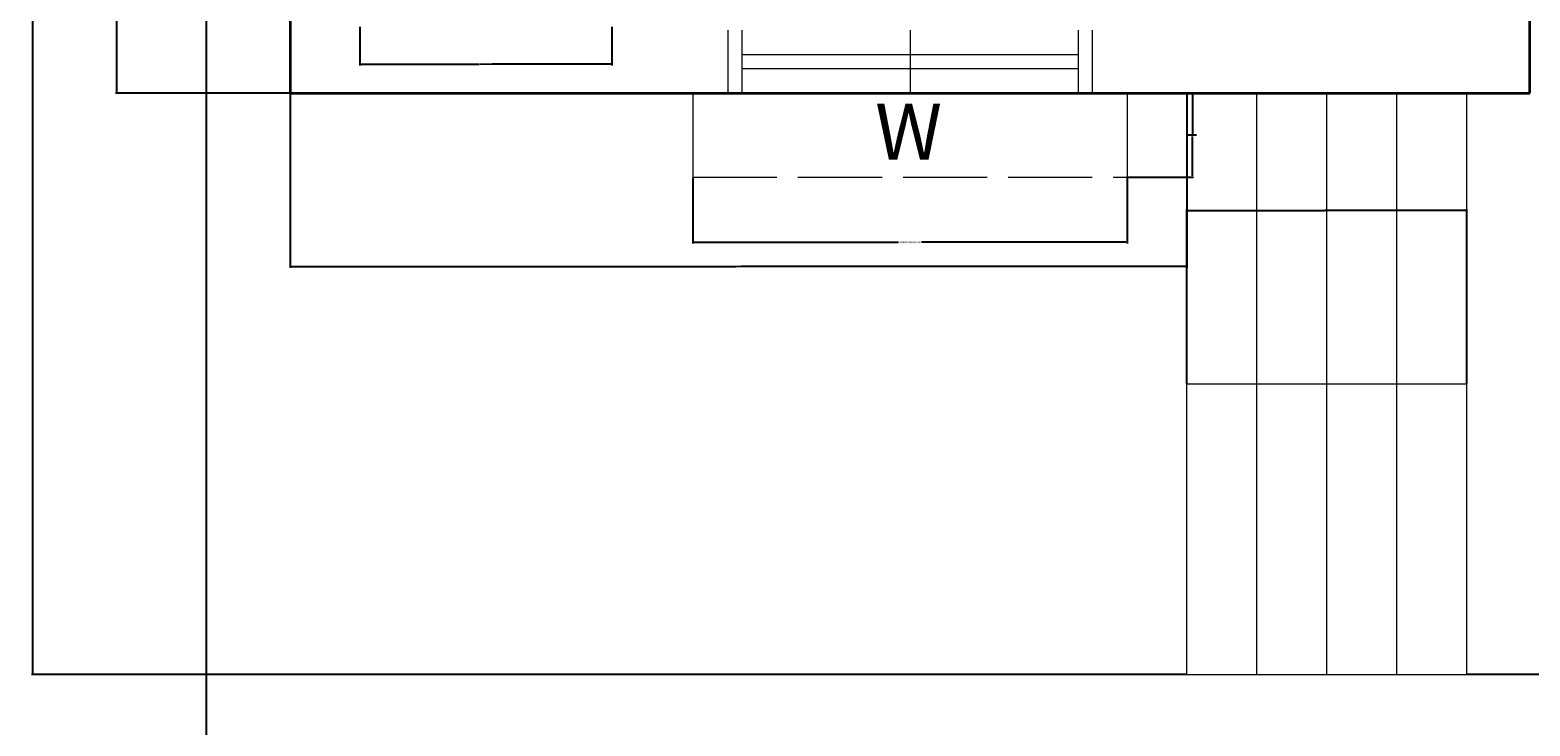
# Model space of a CAD drawing. Units: inches. Extents: x -35 to 832, y -515 to 219.
# Tile 2 of 7: x -35 to 179, y -262 to -163. Entities that reach past the tile are written whole.
import ezdxf

# ---------------------------------------------------------------- set-up
doc = ezdxf.new("R2010")
doc.units = ezdxf.units.IN
doc.header["$MEASUREMENT"] = 0
doc.linetypes.add('ACAD_ISO02W100', pattern=[15, 12, -3])
for name, color, linetype, lineweight in [('A-ANNO-TEXT', 7, 'Continuous', 18), ('A-FLOR', 7, 'Continuous', 25), ('A-FLOR-STRS', 2, 'Continuous', 18), ('A-GLAZ', 2, 'Continuous', 18), ('A-GLAZ-OVHD', 2, 'ACAD_ISO02W100', 13), ('A-WALL', 10, 'Continuous', 35), ('S-ANNO-DIMS', 2, 'Continuous', 18)]:
    doc.layers.add(name, color=color, linetype=linetype, lineweight=lineweight)
doc.styles.get("Standard").update_dxf_attribs({"font": 'arial.ttf'})
doc.dimstyles.get("Standard").update_dxf_attribs({"dimtxt": 0.18, "dimasz": 0.18, "dimexe": 0.18, "dimexo": 0.0625, "dimgap": 0.09, "dimtad": 0, "dimtih": 1, "dimtoh": 1, "dimdec": 1, "dimzin": 0, "dimdsep": 46, "dimlunit": 4, "dimtxsty": 'Standard', "dimcen": 0.09, "dimclrd": 211, "dimclre": 4, "dimclrt": 3, "dimadec": 0, "dimazin": 0, "dimtfac": 0.5, "dimtdec": 1, "dimtofl": 0, "dimtmove": 0, "dimatfit": 3, "dimfxl": 1, "dimtfill": 2, "dimtfillclr": 61, "dimtolj": 1, "dimtzin": 0, "dimarcsym": 0})

# ---------------------------------------------------------------- blocks, each defined once
blk = doc.blocks.new('WIN-48')
for p, q in [((0, 9), (0, 0)), ((2, 9), (2, 0)), ((26, 9), (26, 0)), ((50, 9), (50, 0)), ((52, 9), (52, 0)), ((2, 5.5), (50, 5.5)), ((2, 3.5), (50, 3.5))]:
    blk.add_line(p, q)
blk = doc.blocks.new('WIN-48-HOOD')
for p, q in [((5, 12), (0, 12)), ((0, 12), (0, 0)), ((57, 12), (62, 12)), ((62, 12), (62, 0)), ((0, 0), (62, 0))]:
    blk.add_line(p, q)
blk = doc.blocks.new('*D63')
at = {"layer": 'Defpoints', "color": 0, "transparency": 16777216}
for p in [(59.3, -183.95), (121.3, -183.95), (121.3, -193.25)]:
    blk.add_point(p, dxfattribs=at)
at = {"layer": 'S-ANNO-DIMS', "color": 4, "lineweight": -2, "transparency": 16777216}
for p, q in [((59.3, -184.01), (59.3, -193.43)), ((121.3, -184.01), (121.3, -193.43))]:
    blk.add_line(p, q, dxfattribs=at)
at = {"layer": 'S-ANNO-DIMS', "color": 211, "lineweight": -2, "transparency": 16777216}
for p, q in [((59.48, -193.25), (88.66, -193.25)), ((121.12, -193.25), (91.94, -193.25))]:
    blk.add_line(p, q, dxfattribs=at)
at = {"layer": 'S-ANNO-DIMS', "color": 211, "transparency": 16777216}
for points in [[(59.48, -193.22), (59.48, -193.28), (59.3, -193.25)], [(121.12, -193.22), (121.12, -193.28), (121.3, -193.25)]]:
    blk.add_solid(points, dxfattribs=at)
at = {"layer": 'S-ANNO-DIMS', "color": 3, "transparency": 16777216, "insert": (90.3, -193.25), "char_height": 0.18, "attachment_point": 5, "bg_fill": 1, "box_fill_scale": 1.25, "bg_fill_color": 61, "bg_fill_transparency": 0}
blk.add_mtext('\\A1;WINDOW HOOD 5\'-2" TYP.', dxfattribs=at)
blk = doc.blocks.new('*D64')
at = {"layer": 'Defpoints', "color": 0, "transparency": 16777216}
for p in [(121.3, -171.95), (130.6, -171.95), (121.3, -183.95)]:
    blk.add_point(p, dxfattribs=at)
at = {"layer": 'S-ANNO-DIMS', "color": 4, "lineweight": -2, "transparency": 16777216}
for p, q in [((121.36, -171.95), (130.78, -171.95)), ((121.36, -183.95), (130.78, -183.95))]:
    blk.add_line(p, q, dxfattribs=at)
at = {"layer": 'S-ANNO-DIMS', "color": 211, "lineweight": -2, "transparency": 16777216}
for p, q in [((130.6, -172.13), (130.6, -177.77)), ((130.6, -183.77), (130.6, -178.13))]:
    blk.add_line(p, q, dxfattribs=at)
at = {"layer": 'S-ANNO-DIMS', "color": 211, "transparency": 16777216}
for points in [[(130.57, -172.13), (130.63, -172.13), (130.6, -171.95)], [(130.57, -183.77), (130.63, -183.77), (130.6, -183.95)]]:
    blk.add_solid(points, dxfattribs=at)
at = {"layer": 'S-ANNO-DIMS', "color": 3, "transparency": 16777216, "insert": (130.6, -177.95), "char_height": 0.18, "attachment_point": 5, "bg_fill": 1, "box_fill_scale": 1.25, "bg_fill_color": 61, "bg_fill_transparency": 0}
blk.add_mtext('\\A1;1\'-0" TYP.', dxfattribs=at)
blk = doc.blocks.new('*D81')
at = {"layer": 'Defpoints', "color": 0, "transparency": 16777216}
for p in [(11.74, -162.42), (47.74, -162.42), (47.74, -167.82)]:
    blk.add_point(p, dxfattribs=at)
at = {"layer": 'S-ANNO-DIMS', "color": 4, "lineweight": -2, "transparency": 16777216}
for p, q in [((11.74, -162.48), (11.74, -168)), ((47.74, -162.48), (47.74, -168))]:
    blk.add_line(p, q, dxfattribs=at)
at = {"layer": 'S-ANNO-DIMS', "color": 211, "lineweight": -2, "transparency": 16777216}
for p, q in [((11.92, -167.82), (28.83, -167.82)), ((47.56, -167.82), (30.65, -167.82))]:
    blk.add_line(p, q, dxfattribs=at)
at = {"layer": 'S-ANNO-DIMS', "color": 211, "transparency": 16777216}
for points in [[(11.92, -167.79), (11.92, -167.85), (11.74, -167.82)], [(47.56, -167.79), (47.56, -167.85), (47.74, -167.82)]]:
    blk.add_solid(points, dxfattribs=at)
at = {"layer": 'S-ANNO-DIMS', "color": 3, "transparency": 16777216, "insert": (29.74, -167.82), "char_height": 0.18, "attachment_point": 5, "bg_fill": 1, "box_fill_scale": 1.25, "bg_fill_color": 61, "bg_fill_transparency": 0}
blk.add_mtext('\\A1;CABINET 3\'-0"', dxfattribs=at)
blk = doc.blocks.new('*D107')
at = {"layer": 'Defpoints', "color": 0, "transparency": 16777216}
for p in [(1.8, -171.95), (129.8, -171.95), (1.8, -196.7)]:
    blk.add_point(p, dxfattribs=at)
at = {"layer": 'S-ANNO-DIMS', "color": 4, "lineweight": -2, "transparency": 16777216}
for p, q in [((1.8, -172.01), (1.8, -196.88)), ((129.8, -172.01), (129.8, -196.88))]:
    blk.add_line(p, q, dxfattribs=at)
at = {"layer": 'S-ANNO-DIMS', "color": 211, "lineweight": -2, "transparency": 16777216}
for p, q in [((1.98, -196.7), (65.41, -196.7)), ((129.62, -196.7), (66.19, -196.7))]:
    blk.add_line(p, q, dxfattribs=at)
at = {"layer": 'S-ANNO-DIMS', "color": 211, "transparency": 16777216}
for points in [[(1.98, -196.67), (1.98, -196.73), (1.8, -196.7)], [(129.62, -196.67), (129.62, -196.73), (129.8, -196.7)]]:
    blk.add_solid(points, dxfattribs=at)
at = {"layer": 'S-ANNO-DIMS', "color": 3, "transparency": 16777216, "insert": (65.8, -196.7), "char_height": 0.18, "attachment_point": 5, "bg_fill": 1, "box_fill_scale": 1.25, "bg_fill_color": 61, "bg_fill_transparency": 0}
blk.add_mtext('\\A1;10\'-8"', dxfattribs=at)
blk = doc.blocks.new('*D108')
at = {"layer": 'Defpoints', "color": 0, "transparency": 16777216}
for p in [(169.8, -188.7), (129.8, -213.45), (169.8, -213.45)]:
    blk.add_point(p, dxfattribs=at)
at = {"layer": 'S-ANNO-DIMS', "color": 4, "lineweight": -2, "transparency": 16777216}
for p, q in [((129.8, -213.39), (129.8, -188.52)), ((169.8, -213.39), (169.8, -188.52))]:
    blk.add_line(p, q, dxfattribs=at)
at = {"layer": 'S-ANNO-DIMS', "color": 211, "lineweight": -2, "transparency": 16777216}
for p, q in [((129.98, -188.7), (149.47, -188.7)), ((169.62, -188.7), (150.13, -188.7))]:
    blk.add_line(p, q, dxfattribs=at)
at = {"layer": 'S-ANNO-DIMS', "color": 211, "transparency": 16777216}
for points in [[(129.98, -188.67), (129.98, -188.73), (129.8, -188.7)], [(169.62, -188.67), (169.62, -188.73), (169.8, -188.7)]]:
    blk.add_solid(points, dxfattribs=at)
at = {"layer": 'S-ANNO-DIMS', "color": 3, "transparency": 16777216, "insert": (149.8, -188.7), "char_height": 0.18, "attachment_point": 5, "bg_fill": 1, "box_fill_scale": 1.25, "bg_fill_color": 61, "bg_fill_transparency": 0}
blk.add_mtext('\\A1;3\'-4"', dxfattribs=at)
blk = doc.blocks.new('*D109')
at = {"layer": 'Defpoints', "color": 0, "transparency": 16777216}
for p in [(365.8, -100.95), (-10.2, -143.45), (365.8, -279.7)]:
    blk.add_point(p, dxfattribs=at)
at = {"layer": 'S-ANNO-DIMS', "color": 4, "lineweight": -2, "transparency": 16777216}
for p, q in [((365.8, -101.01), (365.8, -279.88)), ((-10.2, -143.51), (-10.2, -279.88))]:
    blk.add_line(p, q, dxfattribs=at)
at = {"layer": 'S-ANNO-DIMS', "color": 211, "lineweight": -2, "transparency": 16777216}
for p, q in [((-10.02, -279.7), (177.4, -279.7)), ((365.62, -279.7), (178.2, -279.7))]:
    blk.add_line(p, q, dxfattribs=at)
at = {"layer": 'S-ANNO-DIMS', "color": 211, "transparency": 16777216}
for points in [[(-10.02, -279.67), (-10.02, -279.73), (-10.2, -279.7)], [(365.62, -279.67), (365.62, -279.73), (365.8, -279.7)]]:
    blk.add_solid(points, dxfattribs=at)
at = {"layer": 'S-ANNO-DIMS', "color": 3, "transparency": 16777216, "insert": (177.8, -279.7), "char_height": 0.18, "attachment_point": 5, "bg_fill": 1, "box_fill_scale": 1.25, "bg_fill_color": 61, "bg_fill_transparency": 0}
blk.add_mtext('\\A1;31\'-4"', dxfattribs=at)
blk = doc.blocks.new('*D110')
at = {"layer": 'Defpoints', "color": 0, "transparency": 16777216}
for p in [(59.3, 194.05), (-34.95, -254.95), (129.8, -254.95)]:
    blk.add_point(p, dxfattribs=at)
at = {"layer": 'S-ANNO-DIMS', "color": 4, "lineweight": -2, "transparency": 16777216}
for p, q in [((59.24, 194.05), (-35.13, 194.05)), ((129.74, -254.95), (-35.13, -254.95))]:
    blk.add_line(p, q, dxfattribs=at)
at = {"layer": 'S-ANNO-DIMS', "color": 211, "lineweight": -2, "transparency": 16777216}
for p, q in [((-34.95, 193.87), (-34.95, -30.27)), ((-34.95, -254.77), (-34.95, -30.63))]:
    blk.add_line(p, q, dxfattribs=at)
at = {"layer": 'S-ANNO-DIMS', "color": 211, "transparency": 16777216}
for points in [[(-34.98, 193.87), (-34.92, 193.87), (-34.95, 194.05)], [(-34.98, -254.77), (-34.92, -254.77), (-34.95, -254.95)]]:
    blk.add_solid(points, dxfattribs=at)
at = {"layer": 'S-ANNO-DIMS', "color": 3, "transparency": 16777216, "insert": (-34.95, -30.45), "char_height": 0.18, "attachment_point": 5, "bg_fill": 1, "box_fill_scale": 1.25, "bg_fill_color": 61, "bg_fill_transparency": 0}
blk.add_mtext('\\A1;37\'-5"', dxfattribs=at)
blk = doc.blocks.new('*D116')
at = {"layer": 'Defpoints', "color": 0, "transparency": 16777216}
for p in [(-22.95, -138.45), (1.8, -138.45), (1.8, -171.95)]:
    blk.add_point(p, dxfattribs=at)
at = {"layer": 'S-ANNO-DIMS', "color": 4, "lineweight": -2, "transparency": 16777216}
for p, q in [((1.74, -138.45), (-23.13, -138.45)), ((1.74, -171.95), (-23.13, -171.95))]:
    blk.add_line(p, q, dxfattribs=at)
at = {"layer": 'S-ANNO-DIMS', "color": 211, "lineweight": -2, "transparency": 16777216}
for p, q in [((-22.95, -138.63), (-22.95, -155.02)), ((-22.95, -171.77), (-22.95, -155.38))]:
    blk.add_line(p, q, dxfattribs=at)
at = {"layer": 'S-ANNO-DIMS', "color": 211, "transparency": 16777216}
for points in [[(-22.98, -138.63), (-22.92, -138.63), (-22.95, -138.45)], [(-22.98, -171.77), (-22.92, -171.77), (-22.95, -171.95)]]:
    blk.add_solid(points, dxfattribs=at)
at = {"layer": 'S-ANNO-DIMS', "color": 3, "transparency": 16777216, "insert": (-22.95, -155.2), "char_height": 0.18, "attachment_point": 5, "bg_fill": 1, "box_fill_scale": 1.25, "bg_fill_color": 61, "bg_fill_transparency": 0}
blk.add_mtext('\\A1;2\'-9 1/2"', dxfattribs=at)

msp = doc.modelspace()

# ---------------------------------------------------------------- linework, layer by layer
at = {"layer": 'A-FLOR'}
msp.add_line((353.8, -254.95), (169.8, -254.95), dxfattribs=at)
at = {"layer": 'A-FLOR-STRS'}
for p, q in [((129.8, -254.95), (129.8, -171.95)), ((139.8, -254.95), (139.8, -171.95)), ((149.8, -254.95), (149.8, -171.95)), ((159.8, -254.95), (159.8, -171.95)), ((169.8, -254.95), (169.8, -171.95)), ((129.8, -213.45), (169.8, -213.45)), ((129.8, -254.95), (169.8, -254.95))]:
    msp.add_line(p, q, dxfattribs=at)
at = {"layer": 'A-WALL'}
for p, q in [((1.8, -52.95), (1.8, -171.95)), ((178.8, -171.95), (178.8, -101.95)), ((1.8, -171.95), (178.8, -171.95))]:
    msp.add_line(p, q, dxfattribs=at)

# ---------------------------------------------------------------- block references
at = {"layer": 'A-GLAZ'}
msp.add_blockref('WIN-48', (64.3, -171.95), dxfattribs=at)
at = {"layer": 'A-GLAZ-OVHD'}
msp.add_blockref('WIN-48-HOOD', (59.3, -183.95), dxfattribs=at)

# ---------------------------------------------------------------- texts
at = {"layer": 'A-ANNO-TEXT'}
msp.add_text('W', height=8, dxfattribs=at).set_placement((85.3, -181.45))

# ---------------------------------------------------------------- dimensions: what is measured, and where the dimension line sits
at = {"layer": 'S-ANNO-DIMS'}
for base, p1, p2, angle, picture, middle in [((-34.95, -254.95), (59.3, 194.05), (129.8, -254.95), 90, '*D110', (-34.95, -30.45)), ((-22.95, -138.45), (1.8, -171.95), (1.8, -138.45), 90, '*D116', (-22.95, -155.2)), ((1.8, -196.7), (129.8, -171.95), (1.8, -171.95), 180, '*D107', (65.8, -196.7))]:
    dim = msp.add_linear_dim(base=base, p1=p1, p2=p2, angle=angle, dimstyle='Standard', override={"dimdec": 1, "dimlfac": 1, "dimrnd": 0, "dimzin": 1, "dimdsep": 46, "dimlunit": 4, "dimfrac": 2}, dxfattribs=at)
    dim.commit()
    dim.dimension.update_dxf_attribs({"geometry": picture, "text_midpoint": middle})
for base, p1, p2, picture, middle in [((365.8, -279.7), (-10.2, -143.45), (365.8, -100.95), '*D109', (177.8, -279.7)), ((169.8, -188.7), (129.8, -213.45), (169.8, -213.45), '*D108', (149.8, -188.7))]:
    dim = msp.add_linear_dim(base=base, p1=p1, p2=p2, dimstyle='Standard', override={"dimdec": 1, "dimlfac": 1, "dimrnd": 0, "dimzin": 1, "dimdsep": 46, "dimlunit": 4, "dimfrac": 2}, dxfattribs=at)
    dim.commit()
    dim.dimension.update_dxf_attribs({"geometry": picture, "text_midpoint": middle})
for base, p1, p2, text, picture, middle in [((47.74, -167.82), (11.74, -162.42), (47.74, -162.42), 'CABINET <>', '*D81', (29.74, -167.82)), ((121.3, -193.25), (59.3, -183.95), (121.3, -183.95), 'WINDOW HOOD <> TYP.', '*D63', (90.3, -193.25))]:
    dim = msp.add_linear_dim(base=base, p1=p1, p2=p2, text=text, dimstyle='Standard', override={"dimdec": 1, "dimlfac": 1, "dimrnd": 0, "dimzin": 1, "dimdsep": 46, "dimlunit": 4, "dimfrac": 2}, dxfattribs=at)
    dim.commit()
    dim.dimension.update_dxf_attribs({"geometry": picture, "text_midpoint": middle})
dim = msp.add_linear_dim(base=(130.6, -171.95), p1=(121.3, -183.95), p2=(121.3, -171.95), angle=90, text='<> TYP.', dimstyle='Standard', override={"dimdec": 1, "dimlfac": 1, "dimrnd": 0, "dimzin": 1, "dimdsep": 46, "dimlunit": 4, "dimfrac": 2}, dxfattribs=at)
dim.commit()
dim.dimension.update_dxf_attribs({"geometry": '*D64', "text_midpoint": (130.6, -177.95)})

doc.saveas('drawing.dxf')
